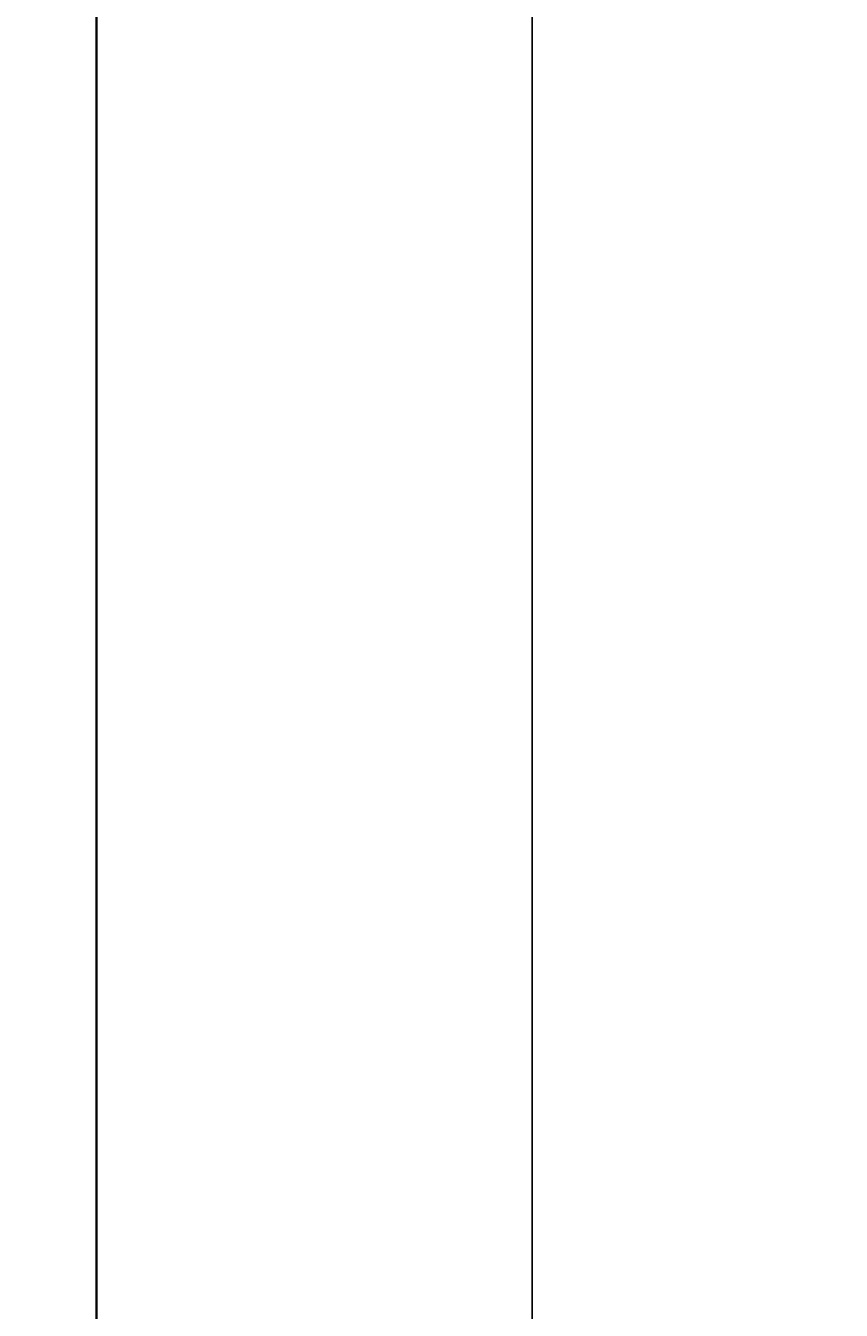
# Model space of a CAD drawing. Units: inches. Extents: x 3731 to 4318, y 1310 to 2388.
# Tile 10 of 57: x 3944 to 3985, y 1398 to 1463. Entities that reach past the tile are written whole.
import ezdxf

# ---------------------------------------------------------------- set-up
doc = ezdxf.new("R2010")
doc.units = ezdxf.units.IN
doc.layers.add('A-ANNO-DIMS', color=2, linetype='Continuous', lineweight=18)
doc.layers.add('A-WALL', color=7, linetype='Continuous', lineweight=35)
doc.styles.get("Standard").update_dxf_attribs({"font": 'arial.ttf'})
doc.dimstyles.get("Standard").update_dxf_attribs({"dimtxt": 0.18, "dimasz": 0.18, "dimexe": 0.18, "dimexo": 0.0625, "dimgap": 0.09, "dimtad": 0, "dimtih": 1, "dimtoh": 1, "dimdec": 4, "dimzin": 0, "dimdsep": 46, "dimtxsty": 'Standard', "dimcen": 0.09, "dimadec": 0, "dimazin": 0, "dimtfac": 1, "dimtdec": 4, "dimtofl": 0, "dimtmove": 0, "dimatfit": 3, "dimfxl": 1, "dimtolj": 1, "dimtzin": 0, "dimarcsym": 0})

# ---------------------------------------------------------------- blocks, each defined once
blk = doc.blocks.new('*D32')
at = {"layer": 'A-ANNO-DIMS', "color": 0, "lineweight": -2, "transparency": 16777216}
for p, q in [((4269.211, 1592.319), (4269.211, 1310.251)), ((3835.209, 1359.319), (3835.209, 1310.251)), ((3835.389, 1310.431), (4051.918, 1310.431)), ((4269.031, 1310.431), (4052.502, 1310.431))]:
    blk.add_line(p, q, dxfattribs=at)
at = {"layer": 'A-ANNO-DIMS', "color": 0, "transparency": 16777216}
for points in [[(3835.389, 1310.461), (3835.389, 1310.401), (3835.209, 1310.431)], [(4269.031, 1310.461), (4269.031, 1310.401), (4269.211, 1310.431)]]:
    blk.add_solid(points, dxfattribs=at)
at = {"layer": 'Defpoints', "color": 0, "transparency": 16777216}
for p in [(4269.211, 1592.382), (3835.209, 1359.382), (4269.211, 1310.431)]:
    blk.add_point(p, dxfattribs=at)
at = {"layer": 'A-ANNO-DIMS', "color": 0, "transparency": 16777216, "insert": (4052.21, 1310.431), "char_height": 0.18, "attachment_point": 5}
blk.add_mtext('\\A1;434', dxfattribs=at)
blk = doc.blocks.new('*D44')
at = {"layer": 'A-ANNO-DIMS', "color": 0, "lineweight": -2, "transparency": 16777216}
for p, q in [((3969.209, 1874.319), (3969.209, 1310.251)), ((4029.209, 1874.319), (4029.209, 1310.251)), ((3969.389, 1310.431), (3998.99, 1310.431)), ((4029.029, 1310.431), (3999.428, 1310.431))]:
    blk.add_line(p, q, dxfattribs=at)
at = {"layer": 'A-ANNO-DIMS', "color": 0, "transparency": 16777216}
for points in [[(3969.389, 1310.461), (3969.389, 1310.401), (3969.209, 1310.431)], [(4029.029, 1310.461), (4029.029, 1310.401), (4029.209, 1310.431)]]:
    blk.add_solid(points, dxfattribs=at)
at = {"layer": 'Defpoints', "color": 0, "transparency": 16777216}
for p in [(3969.209, 1874.382), (4029.209, 1874.382), (4029.209, 1310.431)]:
    blk.add_point(p, dxfattribs=at)
at = {"layer": 'A-ANNO-DIMS', "color": 0, "transparency": 16777216, "insert": (3999.209, 1310.431), "char_height": 0.18, "attachment_point": 5}
blk.add_mtext('\\A1;60', dxfattribs=at)

msp = doc.modelspace()

# ---------------------------------------------------------------- linework, layer by layer
at = {"layer": 'A-WALL'}
msp.add_line((3947.211, 1484.382), (3947.211, 1364.382), dxfattribs=at)

# ---------------------------------------------------------------- dimensions: what is measured, and where the dimension line sits
at = {"layer": 'A-ANNO-DIMS'}
for base, p1, p2, picture, middle in [((4029.209, 1310.431), (3969.209, 1874.382), (4029.209, 1874.382), '*D44', (3999.209, 1310.431)), ((4269.211, 1310.431), (3835.209, 1359.382), (4269.211, 1592.382), '*D32', (4052.21, 1310.431))]:
    dim = msp.add_linear_dim(base=base, p1=p1, p2=p2, dimstyle='Standard', override={"dimdec": 0, "dimlfac": 1, "dimrnd": 0, "dimzin": 0, "dimdsep": 46, "dimlunit": 2}, dxfattribs=at)
    dim.commit()
    dim.dimension.update_dxf_attribs({"geometry": picture, "text_midpoint": middle})

doc.saveas('drawing.dxf')
